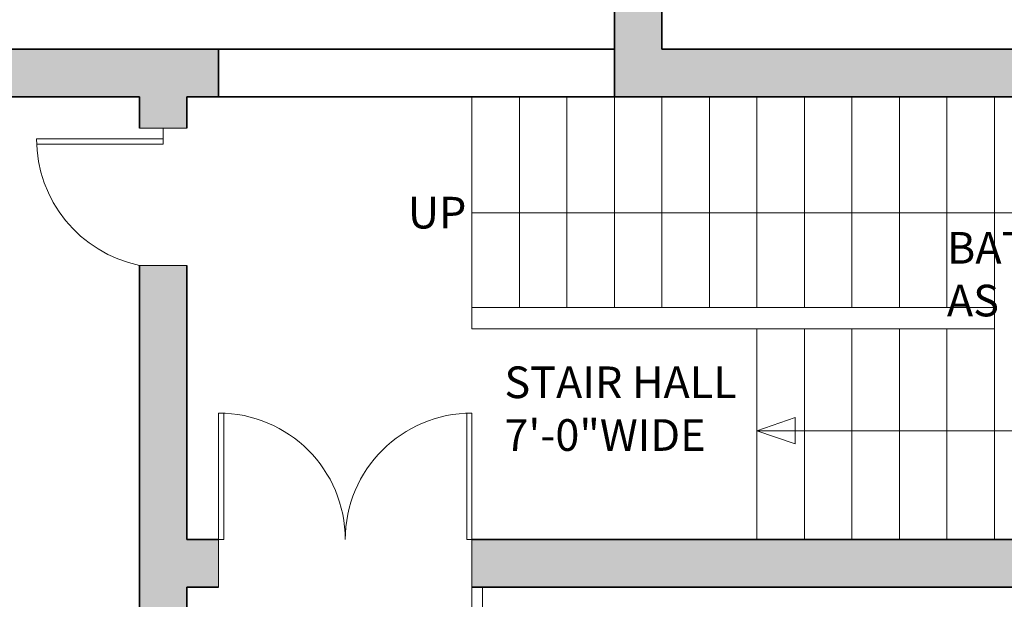
# Model space of a CAD drawing. Units: inches. Extents: x -9 to 646, y -802 to 47.
# Tile 10 of 17: x 326 to 512, y -522 to -412. Entities that reach past the tile are written whole.
import ezdxf

# ---------------------------------------------------------------- set-up
doc = ezdxf.new("R2010")
doc.units = ezdxf.units.IN
doc.header["$MEASUREMENT"] = 0
for name, color, linetype, lineweight in [('A-ANNO-SYMB', 7, 'Continuous', 13), ('A-ANNO-TEXT', 7, 'Continuous', 18), ('A-AREA-IDEN', 7, 'Continuous', 18), ('A-DOOR', 4, 'Continuous', 18), ('A-FLOR-STRS', 7, 'Continuous', 18), ('A-WALL', 7, 'Continuous', 35), ('A-WALL-PATT', 5, 'Continuous', 9)]:
    doc.layers.add(name, color=color, linetype=linetype, lineweight=lineweight)
doc.styles.get("Standard").update_dxf_attribs({"font": 'arial.ttf'})

# ---------------------------------------------------------------- blocks, each defined once
blk = doc.blocks.new('DOOR-LEAF-24-WALL9')
for p, q in [((0, 0), (0, 24)), ((1, 0), (1, 24)), ((0, 0), (1, 0))]:
    blk.add_line(p, q)
blk.add_arc((0, -0.52), 24.52, 11.8123, 90)

msp = doc.modelspace()

# ---------------------------------------------------------------- hatches: boundary and pattern name
at = {"layer": 'A-WALL-PATT'}
h = msp.add_hatch(color=256, dxfattribs=at)
h.dxf.hatch_style = 1
h.paths.add_polyline_path([(73.4, -418.07), (63.37, -418.07), (63.37, -487.07), (63.35, -496.07), (67.87, -496.07), (67.87, -427.07), (73.4, -427.07)])
h.paths.add_polyline_path([(73.87, -487.07), (67.87, -487.07), (67.87, -496.07), (73.87, -496.07)])
h.paths.add_polyline_path([(39.37, -496.07), (39.35, -496.07), (39.35, -487.07), (30.37, -487.07), (30.37, -646.07), (69.62, -646.07), (69.62, -637.07), (39.37, -637.07)])
h.paths.add_polyline_path([(158.27, -637.07), (105.62, -637.07), (105.62, -646.07), (158.27, -646.07)])
h.paths.add_polyline_path([(286.47, -637.07), (194.27, -637.07), (194.27, -646.07), (286.47, -646.07)])
h.paths.add_polyline_path([(357.37, -552.07), (352.87, -552.07), (348.37, -552.07), (348.37, -637.07), (322.47, -637.07), (322.47, -646.07), (357.37, -646.07)])
h.paths.add_polyline_path([(357.37, -459.07), (352.87, -459.07), (348.37, -459.07), (348.37, -526.07), (357.37, -526.07), (357.37, -520.07), (363.37, -520.07), (363.37, -511.07), (357.37, -511.07)], flags=17)
h.paths.add_polyline_path([(39.37, -262.07), (213.37, -262.07), (213.37, -268.07), (222.37, -268.07), (222.37, -247.07), (213.37, -247.07), (213.37, -253.07), (39.37, -253.07), (39.37, -1.07), (222.37, -1.07), (222.37, 7.93), (30.37, 7.93), (30.37, -427.07), (39.36, -427.07), (39.36, -418.07)])
h.paths.add_polyline_path([(570.37, -149.32), (561.37, -149.32), (561.37, -161.07), (433.37, -161.07), (433.37, -165.57), (433.37, -170.07), (438.37, -170.07), (438.37, -176.07), (447.37, -176.07), (447.37, -170.07), (561.37, -170.07), (561.37, -229.57), (570.37, -229.57)])
h.paths.add_polyline_path([(570.37, -289.57), (561.37, -289.57), (561.37, -349.07), (479.37, -349.07), (479.37, -353.57), (479.37, -358.07), (561.37, -358.07), (561.37, -418.07), (447.37, -418.07), (447.37, -358.07), (453.37, -358.07), (453.37, -349.07), (447.37, -349.07), (447.37, -202.07), (442.87, -202.07), (438.37, -202.07), (438.37, -427.07), (561.37, -427.07), (561.37, -451.07), (570.37, -451.07)])
h.paths.add_polyline_path([(570.37, -496.07), (570.37, -487.07), (561.37, -487.07), (561.37, -511.07), (411.37, -511.07), (411.37, -515.57), (411.37, -520.07), (570.37, -520.07)])
h = msp.add_hatch(color=256, dxfattribs=at)
h.dxf.hatch_style = 1
h.paths.add_polyline_path([(363.37, -418.07), (222.37, -418.07), (222.37, -294.07), (217.87, -294.07), (213.37, -294.07), (213.37, -418.07), (101.62, -418.07), (101.62, -427.07), (135.37, -427.07), (135.37, -487.07), (99.87, -487.07), (99.87, -491.57), (99.87, -496.07), (135.37, -496.07), (135.37, -568.07), (39.37, -568.07), (39.37, -496.07), (39.35, -496.07), (39.35, -487.07), (30.37, -487.07), (30.37, -646.07), (69.62, -646.07), (69.62, -637.07), (39.37, -637.07), (39.37, -577.07), (135.37, -577.07), (135.37, -605.07), (137.62, -605.07), (139.87, -605.07), (139.87, -427.07), (348.37, -427.07), (348.37, -433.07), (357.37, -433.07), (357.37, -427.07), (363.37, -427.07)])
h = msp.add_hatch(color=256, dxfattribs=at)
h.dxf.hatch_style = 1
h.paths.add_polyline_path([(570.37, -496.07), (570.37, -487.07), (561.37, -487.07), (561.37, -511.07), (411.37, -511.07), (411.37, -515.57), (411.37, -520.07), (570.37, -520.07)])

# ---------------------------------------------------------------- linework, layer by layer
at = {"layer": 'A-ANNO-SYMB'}
for p, q in [((411.37, -449.07), (523.2, -449.07)), ((465.37, -490.46), (472.6, -487.9)), ((472.6, -487.9), (472.6, -492.92)), ((523.2, -490.46), (465.37, -490.46)), ((472.6, -492.92), (465.37, -490.46))]:
    msp.add_line(p, q, dxfattribs=at)
at = {"layer": 'A-DOOR'}
for p, q in [((348.37, -433.07), (357.37, -433.07)), ((352.87, -433.07), (352.87, -435.07)), ((352.87, -459.07), (348.37, -459.07)), ((352.87, -459.07), (357.37, -459.07)), ((363.37, -511.07), (363.37, -487.07)), ((364.37, -511.07), (364.37, -487.07)), ((410.37, -511.07), (410.37, -487.07)), ((411.37, -511.07), (411.37, -487.07)), ((363.37, -520.07), (363.37, -511.07)), ((364.37, -511.07), (363.37, -511.07)), ((410.37, -511.07), (411.37, -511.07)), ((411.37, -515.57), (411.37, -511.07)), ((411.37, -515.57), (411.37, -520.07))]:
    msp.add_line(p, q, dxfattribs=at)
for centre, start, end in [((363.37, -511.07), 0, 90), ((411.37, -511.07), 90, 180)]:
    msp.add_arc(centre, 24, start, end, dxfattribs=at)
at = {"layer": 'A-FLOR-STRS'}
for p, q in [((411.37, -427.07), (411.37, -471.07)), ((420.37, -427.07), (420.37, -467.07)), ((429.37, -427.07), (429.37, -467.07)), ((438.37, -427.07), (438.37, -467.07)), ((447.37, -427.07), (447.37, -467.07)), ((456.37, -427.07), (456.37, -467.07)), ((465.37, -427.07), (465.37, -467.07)), ((474.37, -427.07), (474.37, -467.07)), ((483.37, -427.07), (483.37, -467.07)), ((492.37, -427.07), (492.37, -467.07)), ((501.37, -427.07), (501.37, -467.07)), ((510.37, -427.07), (510.37, -511.07)), ((510.37, -467.07), (411.37, -467.07)), ((510.37, -471.07), (411.37, -471.07)), ((465.37, -471.07), (465.37, -511.07)), ((474.37, -471.07), (474.37, -511.07)), ((483.37, -471.07), (483.37, -511.07)), ((492.37, -471.07), (492.37, -511.07)), ((501.37, -471.07), (501.37, -511.07)), ((411.37, -487.07), (411.37, -511.07)), ((411.37, -520.07), (411.37, -646.07)), ((413.37, -520.07), (413.37, -646.07))]:
    msp.add_line(p, q, dxfattribs=at)
at = {"layer": 'A-WALL'}
for p, q in [((438.37, -202.07), (438.37, -427.07)), ((447.37, -358.07), (447.37, -418.07)), ((222.37, -418.07), (438.37, -418.07)), ((363.37, -427.07), (363.37, -418.07)), ((447.37, -418.07), (561.37, -418.07)), ((139.87, -427.07), (348.37, -427.07)), ((348.37, -427.07), (348.37, -433.07)), ((357.37, -427.07), (357.37, -433.07)), ((357.37, -427.07), (561.37, -427.07)), ((348.37, -459.07), (348.37, -526.07)), ((357.37, -459.07), (357.37, -511.07)), ((357.37, -511.07), (363.37, -511.07)), ((411.37, -511.07), (561.37, -511.07)), ((357.37, -520.07), (363.37, -520.07)), ((357.37, -520.07), (363.37, -520.07)), ((357.37, -520.07), (357.37, -526.07)), ((411.37, -520.07), (570.37, -520.07))]:
    msp.add_line(p, q, dxfattribs=at)

# ---------------------------------------------------------------- block references
at = {"layer": 'A-DOOR', "extrusion": (0, 0, -1), "zscale": -1, "rotation": 270.0000000000002}
msp.add_blockref('DOOR-LEAF-24-WALL9', (-352.87, -435.07), dxfattribs=at)

# ---------------------------------------------------------------- texts
at = {"layer": 'A-ANNO-TEXT', "insert": (399.23, -446.06), "char_height": 6, "attachment_point": 1}
msp.add_mtext_dynamic_manual_height_columns('UP', width=3.8078, gutter_width=1, heights=[0], dxfattribs=at)
at = {"layer": 'A-AREA-IDEN', "char_height": 6, "attachment_point": 1}
for s, insert in [('BATH\\PAS PER SITE', (501.37, -452.73)), ('STAIR HALL\\P7\'-0"WIDE', (417.52, -478.23))]:
    msp.add_mtext(s, dxfattribs=dict(at, insert=insert))

doc.saveas('drawing.dxf')
